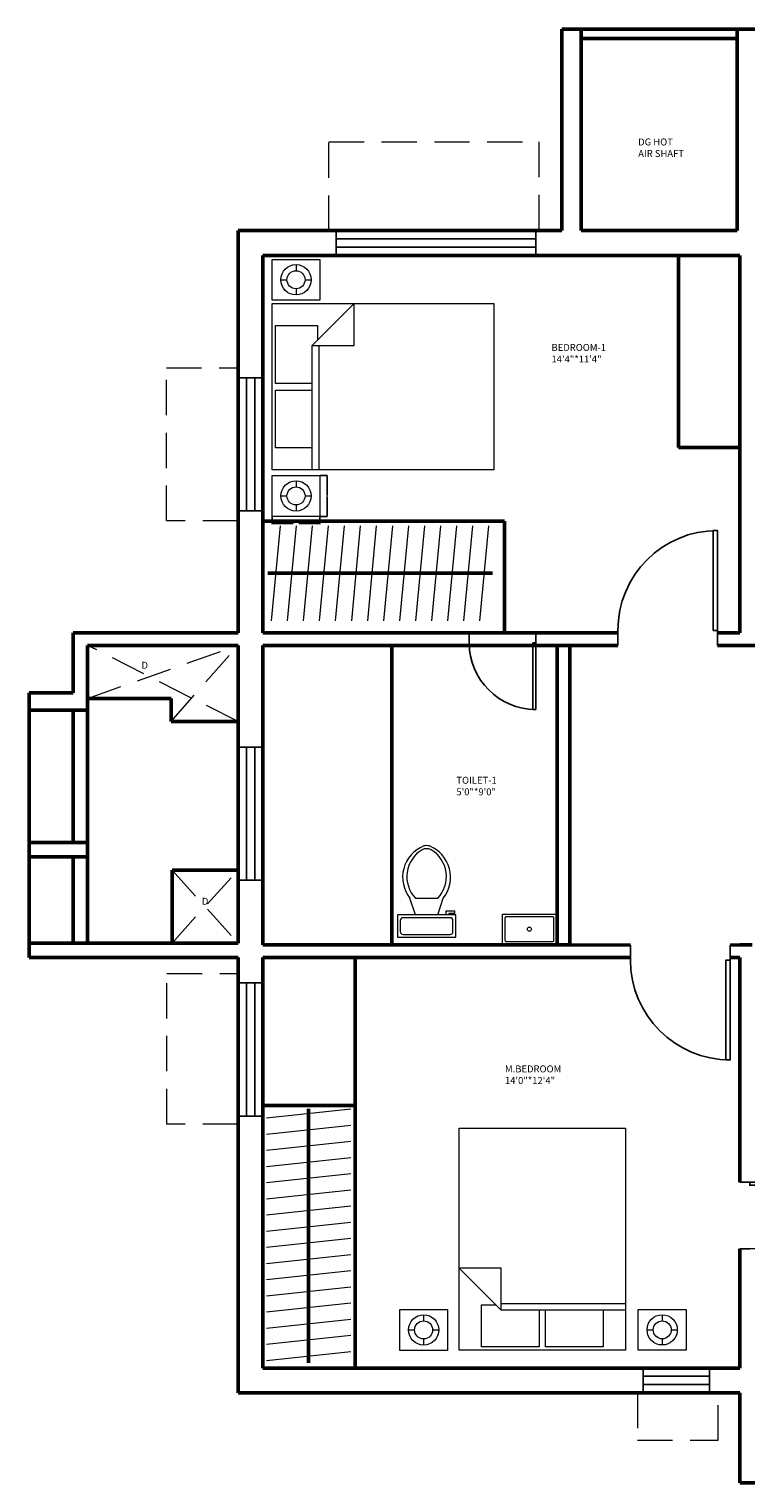
# Model space of a CAD drawing. Units: inches. Extents: x 291 to 2631, y 456 to 2623.
# Tile 1 of 22: x 291 to 550, y 480 to 1004. Entities that reach past the tile are written whole.
import ezdxf

# ---------------------------------------------------------------- set-up
doc = ezdxf.new("R2010")
doc.units = ezdxf.units.IN
doc.linetypes.add('DASHED', pattern=[19.05, 12.7, -6.35])
for name, color, linetype, lineweight in [('A-ANNO-DIMS', 2, 'Continuous', 18), ('A-ANNO-TEXT', 3, 'Continuous', 25), ('A-AREA-IDEN', 7, 'Continuous', 25), ('A-DOOR', 3, 'Continuous', 25), ('A-FLOR-FIXT', 9, 'Continuous', 18), ('A-FLOR-OVHD', 1, 'DASHED', 18), ('A-FURN', 8, 'Continuous', 18), ('A-GLAZ', 4, 'Continuous', 25), ('A-WALL', 7, 'Continuous', 50)]:
    doc.layers.add(name, color=color, linetype=linetype, lineweight=lineweight)
doc.styles.get("Standard").update_dxf_attribs({"font": 'arial.ttf'})
doc.dimstyles.get("Standard").update_dxf_attribs({"dimtxt": 0.18, "dimasz": 0.18, "dimexe": 0.18, "dimexo": 0.0625, "dimgap": 0.09, "dimtad": 0, "dimtih": 1, "dimtoh": 1, "dimdec": 4, "dimzin": 0, "dimdsep": 46, "dimtxsty": 'Standard', "dimcen": 0.09, "dimadec": 0, "dimazin": 0, "dimtfac": 1, "dimtdec": 4, "dimtofl": 0, "dimtmove": 0, "dimatfit": 3, "dimfxl": 1, "dimtolj": 1, "dimtzin": 0, "dimarcsym": 0})

# ---------------------------------------------------------------- blocks, each defined once
blk = doc.blocks.new('*U2')
for p, q in [((0, 0), (0, -6)), ((40, 0), (40, -6))]:
    blk.add_line(p, q)
blk.add_lwpolyline([(0, 0), (0, 40), (1.75, 40), (1.75, 0)], close=True)
blk.add_arc((0, 0), 40, 0, 90)
blk = doc.blocks.new('Bed - Queen')
for p, q in [((0, -80.00003), (0, 0)), ((0, 0), (59.99999, 0)), ((59.99999, 0), (59.99999, -80.00003)), ((7.99999, -1.2), (28.79998, -1.2)), ((7.99999, -14.4), (7.99999, -1.2)), ((28.79998, -1.2), (28.79998, -14.4)), ((31.19999, -1.2), (51.99999, -1.2)), ((31.19999, -14.4), (31.19999, -1.2)), ((51.99999, -1.2), (51.99999, -16.4)), ((0, -14.4), (44.8, -14.4)), ((59.99999, -29.6), (44.8, -14.4)), ((44.8, -14.4), (44.8, -29.6)), ((44.8, -16.8), (0, -16.8)), ((51.99999, -16.4), (46.79936, -16.4)), ((44.8, -29.6), (59.99999, -29.6)), ((59.99999, -80.00003), (0, -80.00003))]:
    blk.add_line(p, q)
blk = doc.blocks.new('Toilet - top')
for p, q in [((9.5, -6), (9.5, -2)), ((-10, -8.5), (-8, -8.5)), ((-10, -9.5), (-10, -8.5)), ((-7, -9.5), (-10, -9.5)), ((-8, -8.5), (-8, -8)), ((-7, -8), (-7, -9.5)), ((-4, -8), (-6, -14)), ((4, -8), (6, -14)), ((4, -14), (-4, -14))]:
    blk.add_line(p, q)
blk.add_lwpolyline([(10.5, -8), (10.5, 0), (-10.5, 0), (-10.5, -8)], close=True)
for points in [[(-9.5, -2), (-9.5, -6)], [(8.5, -1), (-8.5, -1)], [(-8.5, -7), (8.5, -7)]]:
    blk.add_lwpolyline(points)
for centre, radius, start, end in [((-8.62, -1.88), 0.884, 81.8699, 188.1301), ((8.62, -1.88), 0.884, 351.8699, 98.1301), ((-8.62, -6.12), 0.884, 171.8699, 278.1301), ((8.62, -6.12), 0.884, 261.8699, 8.1301), ((3.52, -21.58), 12.17, 141.4691, 247.9714), ((4.2, -21.82), 11.33, 136.3677, 238.9468), ((-3.52, -21.58), 12.17, 292.0284, 38.5307), ((-4.2, -21.82), 11.33, 301.053, 43.6321), ((0, -27.88), 4, 245.7318, 294.2682), ((0, -29), 4, 254.8605, 285.1395)]:
    blk.add_arc(centre, radius, start, end)
blk = doc.blocks.new('WIN-1800')
for p, q in [((0, 9), (72, 9)), ((0, 0), (0, 9)), ((0, 6), (72, 6)), ((72, 9), (72, 0)), ((72, 3), (0, 3)), ((72, 0), (0, 0))]:
    blk.add_line(p, q)
blk = doc.blocks.new('WIN-1200')
for p, q in [((0, 0), (0, 48)), ((0, 48), (9, 48)), ((3, 0), (3, 48)), ((6, 48), (6, 0)), ((9, 48), (9, 0)), ((9, 0), (0, 0))]:
    blk.add_line(p, q)
blk = doc.blocks.new('WIN-600')
for p, q in [((24, 9), (0, 9)), ((0, 9), (0, 0)), ((24, 6), (0, 6)), ((24, 0), (24, 9)), ((0, 3), (24, 3)), ((0, 0), (24, 0))]:
    blk.add_line(p, q)
blk = doc.blocks.new('LAMP-B')
for p, q in [((8.62, 12.82), (8.62, 10.61)), ((3.15, 7.36), (5.36, 7.36)), ((11.87, 7.36), (14.08, 7.36)), ((8.62, 4.1), (8.62, 1.89))]:
    blk.add_line(p, q)
blk.add_lwpolyline([(0, 14.71), (17.23, 14.71), (17.23, 0), (0, 0)], close=True)
for radius in [5.46, 3.25]:
    blk.add_circle((8.62, 7.36), radius)
blk = doc.blocks.new('*D42')
at = {"layer": 'A-ANNO-DIMS', "color": 0, "lineweight": -2, "transparency": 16777216}
for p, q in [((378.79, 827.92), (378.79, 825.22)), ((378.97, 825.4), (386.39, 825.4)), ((395.85, 825.4), (388.43, 825.4)), ((396.03, 827.92), (396.03, 825.22))]:
    blk.add_line(p, q, dxfattribs=at)
at = {"layer": 'A-ANNO-DIMS', "color": 0, "transparency": 16777216}
for points in [[(378.97, 825.43), (378.97, 825.37), (378.79, 825.4)], [(395.85, 825.43), (395.85, 825.37), (396.03, 825.4)]]:
    blk.add_solid(points, dxfattribs=at)
at = {"layer": 'DEFPOINTS', "color": 0, "transparency": 16777216}
for p in [(378.79, 827.98), (396.03, 827.98), (396.03, 825.4)]:
    blk.add_point(p, dxfattribs=at)
at = {"layer": 'A-ANNO-DIMS', "color": 0, "transparency": 16777216, "insert": (387.41, 825.4), "char_height": 0.18, "attachment_point": 5}
blk.add_mtext('\\A1;LAMP B 17 TYP.', dxfattribs=at)
blk = doc.blocks.new('*D43')
at = {"layer": 'A-ANNO-DIMS', "color": 0, "lineweight": -2, "transparency": 16777216}
for p, q in [((396.09, 842.69), (398.79, 842.69)), ((398.61, 842.51), (398.61, 835.52)), ((398.61, 828.16), (398.61, 835.15)), ((396.09, 827.98), (398.79, 827.98))]:
    blk.add_line(p, q, dxfattribs=at)
at = {"layer": 'A-ANNO-DIMS', "color": 0, "transparency": 16777216}
for points in [[(398.58, 842.51), (398.64, 842.51), (398.61, 842.69)], [(398.58, 828.16), (398.64, 828.16), (398.61, 827.98)]]:
    blk.add_solid(points, dxfattribs=at)
at = {"layer": 'DEFPOINTS', "color": 0, "transparency": 16777216}
for p in [(396.03, 842.69), (398.61, 842.69), (396.03, 827.98)]:
    blk.add_point(p, dxfattribs=at)
at = {"layer": 'A-ANNO-DIMS', "color": 0, "transparency": 16777216, "insert": (398.61, 835.34), "char_height": 0.18, "attachment_point": 5}
blk.add_mtext('\\A1;15 TYP.', dxfattribs=at)

msp = doc.modelspace()

# ---------------------------------------------------------------- linework, layer by layer
at = {"layer": 'A-FLOR-OVHD'}
for p, q in [((399.26, 930.98), (399.26, 962.98)), ((399.26, 962.98), (475.05, 962.98)), ((475.05, 962.98), (475.05, 930.98)), ((340.64, 826.36), (340.64, 881.52)), ((340.64, 881.52), (366.5, 881.52)), ((366.5, 826.36), (340.64, 826.36)), ((312.24, 762.38), (366.5, 781.48)), ((366.5, 754.02), (312.24, 781.48)), ((342.31, 754.02), (366.5, 781.48)), ((342.69, 700.47), (366.5, 674.14)), ((342.69, 674.14), (366.5, 700.47)), ((340.82, 608.93), (340.82, 663.21)), ((340.82, 663.21), (366.5, 663.21)), ((366.5, 608.93), (340.82, 608.93)), ((510.6, 511.98), (510.6, 494.94)), ((539.71, 494.94), (539.71, 511.98)), ((510.6, 494.94), (539.71, 494.94))]:
    msp.add_line(p, q, dxfattribs=at)
at = {"layer": 'A-FURN'}
for p, q in [((378.59, 790.35), (381.81, 824.62)), ((384.37, 790.35), (387.6, 824.62)), ((390.16, 790.35), (393.38, 824.62)), ((395.94, 790.35), (399.16, 824.62)), ((401.72, 790.35), (404.94, 824.62)), ((407.5, 790.35), (410.72, 824.62)), ((413.28, 790.35), (416.51, 824.62)), ((419.07, 790.35), (422.29, 824.62)), ((424.85, 790.35), (428.07, 824.62)), ((430.63, 790.35), (433.85, 824.62)), ((436.41, 790.35), (439.63, 824.62)), ((442.19, 790.35), (445.42, 824.62)), ((447.97, 790.35), (451.2, 824.62)), ((453.76, 790.35), (456.98, 824.62)), ((376.71, 611.13), (407.15, 614.35)), ((376.71, 611.13), (407.15, 614.35)), ((376.71, 611.13), (407.15, 614.35)), ((376.71, 611.13), (407.15, 614.35)), ((376.71, 611.13), (407.15, 614.35)), ((376.71, 611.13), (407.15, 614.35)), ((376.71, 605.3), (407.15, 608.53)), ((376.71, 599.48), (407.15, 602.7)), ((376.71, 593.65), (407.15, 596.87)), ((376.71, 587.82), (407.15, 591.05)), ((376.71, 582), (407.15, 585.22)), ((376.71, 576.17), (407.15, 579.39)), ((376.71, 570.35), (407.15, 573.57)), ((376.71, 564.52), (407.15, 567.74)), ((376.71, 558.69), (407.15, 561.92)), ((376.71, 552.87), (407.15, 556.09)), ((376.71, 547.04), (407.15, 550.26)), ((376.71, 541.21), (407.15, 544.44)), ((376.71, 535.39), (407.15, 538.61)), ((376.71, 529.56), (407.15, 532.78)), ((376.71, 523.73), (407.15, 526.96))]:
    msp.add_line(p, q, dxfattribs=at)
msp.add_lwpolyline([(481.67, 673.48), (461.86, 673.48), (461.86, 684.59), (481.67, 684.59)], close=True, dxfattribs=at)
msp.add_lwpolyline([(463.4, 683.77), (479.85, 683.77, -0.414214), (480.35, 683.27), (480.35, 675.08, -0.414214), (479.85, 674.58), (463.4, 674.58, -0.414214), (462.9, 675.08), (462.9, 683.27, -0.414214)], format="xyb", close=True, dxfattribs=at)
msp.add_circle((471.62, 679.17), 0.758, dxfattribs=at)
at = {"layer": 'A-WALL'}
for p, q in [((483.37, 930.98), (483.37, 1003.63)), ((483.37, 1003.63), (616.5, 1003.63)), ((490.29, 930.98), (490.29, 1003.63)), ((546.54, 930.98), (546.54, 1003.63)), ((490.29, 1000.21), (546.54, 1000.21)), ((366.5, 862.1), (366.5, 930.98)), ((483.37, 930.98), (366.5, 930.98)), ((546.54, 930.98), (490.29, 930.98)), ((375.5, 862.1), (375.5, 921.98)), ((547.5, 921.98), (375.5, 921.98)), ((525.45, 921.98), (525.45, 852.78)), ((547.5, 862.1), (547.5, 921.98)), ((366.5, 862.1), (366.5, 785.98)), ((375.5, 862.1), (375.5, 785.98)), ((547.5, 862.1), (547.5, 785.98)), ((525.45, 852.78), (547.5, 852.78)), ((375.5, 826.3), (462.58, 826.3)), ((462.58, 826.3), (462.58, 785.98)), ((377.24, 807.49), (458.32, 807.49)), ((307.06, 785.98), (366.5, 785.98)), ((307.06, 764.41), (307.06, 785.98)), ((366.5, 781.48), (312.24, 781.48)), ((312.24, 781.48), (312.24, 674.14)), ((366.5, 781.48), (366.5, 674.14)), ((503.53, 785.98), (375.5, 785.98)), ((375.5, 781.48), (375.5, 673.48)), ((503.53, 781.48), (375.5, 781.48)), ((421.99, 781.48), (421.99, 673.48)), ((481.67, 781.48), (481.67, 673.48)), ((486.17, 781.48), (486.17, 673.48)), ((547.5, 785.98), (539.53, 785.98)), ((702.4, 781.48), (539.53, 781.48)), ((307.06, 764.41), (291.09, 764.41)), ((291.09, 764.41), (291.09, 668.98)), ((312.24, 762.38), (342.31, 762.38)), ((342.31, 762.38), (342.31, 754.02)), ((291.09, 758.14), (312.24, 758.14)), ((307.06, 710.38), (307.06, 758.14)), ((342.31, 754.02), (366.5, 754.02)), ((291.09, 710.38), (312.24, 710.38)), ((291.09, 705.25), (312.24, 705.25)), ((307.06, 674.14), (307.06, 705.25)), ((342.69, 674.14), (342.69, 700.47)), ((342.69, 700.47), (366.5, 700.47)), ((291.09, 674.14), (366.5, 674.14)), ((486.17, 673.48), (375.5, 673.48)), ((508.09, 673.44), (486.17, 673.48)), ((544.09, 673.44), (547.5, 673.48)), ((552, 673.48), (547.5, 673.48)), ((291.09, 668.98), (307.06, 668.98)), ((366.5, 668.98), (307.06, 668.98)), ((366.5, 668.98), (366.5, 511.98)), ((375.5, 668.98), (375.5, 520.98)), ((508.09, 668.98), (375.5, 668.98)), ((408.81, 668.98), (408.81, 520.98)), ((547.5, 668.98), (544.09, 668.98)), ((547.5, 668.98), (547.5, 587.94)), ((375.5, 615.59), (408.81, 615.59)), ((391.93, 614.43), (391.93, 522.81)), ((547.5, 563.94), (547.5, 520.98)), ((547.5, 520.98), (375.5, 520.98)), ((547.5, 511.98), (366.5, 511.98)), ((547.5, 511.98), (547.5, 479.56)), ((547.5, 479.56), (616.5, 479.56))]:
    msp.add_line(p, q, dxfattribs=at)

# ---------------------------------------------------------------- block references
at = {"layer": 'A-DOOR', "xscale": -0.9, "yscale": 0.9, "zscale": 0.9}
msp.add_blockref('*U2', (539.53, 786.88), dxfattribs=at)
at = {"layer": 'A-DOOR'}
for p, xscale, yscale, zscale, rotation in [((473.92, 782.38), 0.6, 0.6, 0.6, 180), ((544.09, 668.04), 0.9, 0.9, 0.9, 180), ((551.1, 587.94), 0.6, 0.6, 0.6, 270)]:
    msp.add_blockref('*U2', p, dxfattribs=dict(at, xscale=xscale, yscale=yscale, zscale=zscale, rotation=rotation))
at = {"layer": 'A-FLOR-FIXT', "rotation": 180}
msp.add_blockref('Toilet - top', (434.54, 676.3), dxfattribs=at)
at = {"layer": 'A-FURN'}
for p in [(378.79, 905.9), (378.79, 827.98), (424.84, 527.35), (510.91, 527.38)]:
    msp.add_blockref('LAMP-B', p, dxfattribs=at)
for p, rotation in [((378.79, 844.73), 90), ((506.29, 527.38), 180)]:
    msp.add_blockref('Bed - Queen', p, dxfattribs=dict(at, rotation=rotation))
at = {"layer": 'A-GLAZ'}
for name, p in [('WIN-1800', (401.93, 921.98)), ('WIN-1200', (366.5, 829.92)), ('WIN-1200', (366.5, 696.81)), ('WIN-1200', (366.5, 611.77))]:
    msp.add_blockref(name, p, dxfattribs=at)
at = {"layer": 'A-GLAZ', "rotation": 180}
msp.add_blockref('WIN-600', (536.64, 520.98), dxfattribs=at)

# ---------------------------------------------------------------- texts
at = {"layer": 'A-ANNO-TEXT', "char_height": 2.5, "attachment_point": 1}
for width, insert in [(3.9307, (331.67, 775.55)), (2.1013, (353.45, 690.47))]:
    msp.add_mtext_dynamic_manual_height_columns('D', width=width, gutter_width=12.5, heights=[0], dxfattribs=dict(at, insert=insert))
at = {"layer": 'A-AREA-IDEN', "char_height": 2.5, "attachment_point": 1}
for s, width, insert in [('DG HOT\\PAIR SHAFT', 48.0812, (510.87, 964.19)), ('BEDROOM-1\\P14\'4"*11\'4"', 57.6603, (479.59, 890.12)), ('TOILET-1\\P5\'0"*9\'0"', 48.8573, (445.27, 734.09)), ('M.BEDROOM\\P14\'0"*12\'4"', 73.6301, (462.8, 630.05))]:
    msp.add_mtext_dynamic_manual_height_columns(s, width=width, gutter_width=12.5, heights=[0], dxfattribs=dict(at, insert=insert))

# ---------------------------------------------------------------- dimensions: what is measured, and where the dimension line sits
at = {"layer": 'A-ANNO-DIMS'}
dim = msp.add_linear_dim(base=(398.61, 842.69), p1=(396.03, 827.98), p2=(396.03, 842.69), angle=90, text='<> TYP.', dimstyle='Standard', override={"dimdec": 0, "dimlfac": 1, "dimrnd": 0, "dimzin": 0, "dimdsep": 46, "dimlunit": 2}, dxfattribs=at)
dim.commit()
dim.dimension.update_dxf_attribs({"geometry": '*D43', "text_midpoint": (398.61, 835.34)})
dim = msp.add_linear_dim(base=(396.03, 825.4), p1=(378.79, 827.98), p2=(396.03, 827.98), text='LAMP B <> TYP.', dimstyle='Standard', override={"dimdec": 0, "dimlfac": 1, "dimrnd": 0, "dimzin": 0, "dimdsep": 46, "dimlunit": 2}, dxfattribs=at)
dim.commit()
dim.dimension.update_dxf_attribs({"geometry": '*D42', "text_midpoint": (387.41, 825.4)})

doc.saveas('drawing.dxf')
